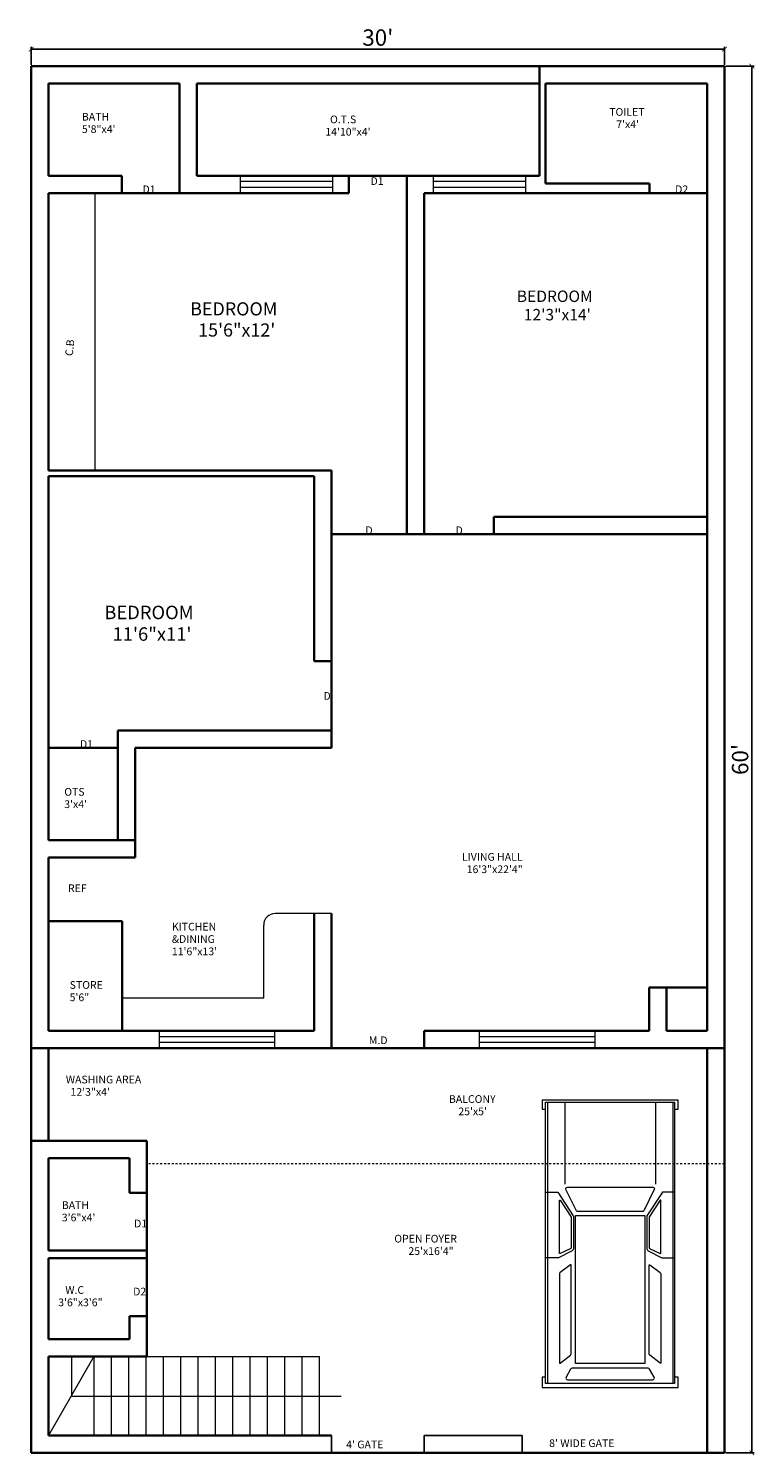
# Model space of a CAD drawing. Units: inches. Extents: x 3799 to 20199, y 1682 to 8087.
# Tile 15 of 30: x 10024 to 10401, y 5781 to 6522. Entities that reach past the tile are written whole.
import ezdxf

# ---------------------------------------------------------------- set-up
doc = ezdxf.new("R2010")
doc.units = ezdxf.units.IN
doc.linetypes.add('JIS_02_1.0', pattern=[2, 1, -1])
for name, color, linetype, lineweight in [('A-ANNO-DIMS', 2, 'Continuous', 18), ('A-ANNO-SYMB', 3, 'Continuous', 18), ('A-ANNO-TEXT', 7, 'Continuous', 18), ('A-AREA-IDEN', 7, 'Continuous', 18), ('A-FLOR-CASE', 32, 'Continuous', 18), ('A-FLOR-STRS', 41, 'Continuous', 18), ('A-GLAZ', 152, 'Continuous', 18), ('A-SITE-OVHD', 8, 'JIS_02_1.0', 18), ('A-SITE-VEHC', 8, 'Continuous', 13), ('A-WALL', 7, 'Continuous', 35), ('C-PROP', 7, 'Continuous', 25)]:
    doc.layers.add(name, color=color, linetype=linetype, lineweight=lineweight)
doc.styles.get("Standard").update_dxf_attribs({"font": 'arial.ttf'})
doc.dimstyles.new('ISO-25', dxfattribs={"dimtxt": 8.5, "dimasz": 2.5, "dimexe": 1.25, "dimexo": 0.625, "dimtad": 1, "dimdec": 0, "dimlunit": 3, "dimtxsty": 'Standard', "dimblk": 'ARCHTICK', "dimcen": 2.5, "dimadec": 0, "dimazin": 0, "dimtfac": 1, "dimtdec": 0, "dimtmove": 0, "dimatfit": 3, "dimfxl": 1, "dimarcsym": 0})

# ---------------------------------------------------------------- blocks, each defined once
blk = doc.blocks.new('_ArchTick')
at = {"color": 0, "linetype": 'ByBlock', "const_width": 0.15}
blk.add_lwpolyline([(-0.5, -0.5), (0.5, 0.5)], dxfattribs=at)
blk = doc.blocks.new('*D197')
at = {"layer": 'A-ANNO-DIMS', "color": 0, "lineweight": -2, "transparency": 16777216}
for p, q in [((10025.38, 6502.81), (10025.38, 6512.16)), ((10385.38, 6510.91), (10025.38, 6510.91)), ((10385.38, 6502.81), (10385.38, 6512.16))]:
    blk.add_line(p, q, dxfattribs=at)
at = {"layer": 'Defpoints', "color": 0, "transparency": 16777216}
for p in [(10025.38, 6510.91), (10025.38, 6502.19), (10385.38, 6502.19)]:
    blk.add_point(p, dxfattribs=at)
at = {"layer": 'A-ANNO-DIMS', "color": 0, "lineweight": -2, "transparency": 16777216, "xscale": 2.5, "yscale": 2.5, "zscale": 2.5, "rotation": 180}
blk.add_blockref('_ArchTick', (10025.38, 6510.91), dxfattribs=at)
at = {"layer": 'A-ANNO-DIMS', "color": 0, "lineweight": -2, "transparency": 16777216, "xscale": 2.5, "yscale": 2.5, "zscale": 2.5}
blk.add_blockref('_ArchTick', (10385.38, 6510.91), dxfattribs=at)
at = {"layer": 'A-ANNO-DIMS', "color": 0, "transparency": 16777216, "insert": (10205.38, 6515.88), "char_height": 8.5, "attachment_point": 5}
blk.add_mtext("30'", dxfattribs=at)
blk = doc.blocks.new('*D198')
at = {"layer": 'A-ANNO-DIMS', "color": 0, "lineweight": -2, "transparency": 16777216}
for p, q in [((10386.01, 6502.19), (10400.8, 6502.19)), ((10399.55, 5782.19), (10399.55, 6502.19)), ((10386.01, 5782.19), (10400.8, 5782.19))]:
    blk.add_line(p, q, dxfattribs=at)
at = {"layer": 'Defpoints', "color": 0, "transparency": 16777216}
for p in [(10385.38, 6502.19), (10399.55, 6502.19), (10385.38, 5782.19)]:
    blk.add_point(p, dxfattribs=at)
at = {"layer": 'A-ANNO-DIMS', "color": 0, "lineweight": -2, "transparency": 16777216, "xscale": 2.5, "yscale": 2.5, "zscale": 2.5}
for p, rotation in [((10399.55, 6502.19), 90), ((10399.55, 5782.19), 270)]:
    blk.add_blockref('_ArchTick', p, dxfattribs=dict(at, rotation=rotation))
at = {"layer": 'A-ANNO-DIMS', "color": 0, "transparency": 16777216, "insert": (10394.59, 6142.19), "char_height": 8.5, "attachment_point": 5, "rotation": 90}
blk.add_mtext("60'", dxfattribs=at)
blk = doc.blocks.new('*U199')
for p, q in [((1.28, 38.87), (175.66, 38.87)), ((1.28, 28.15), (52.13, 28.15)), ((1.28, -28.15), (52.13, -28.15)), ((1.28, -38.87), (175.66, -38.87))]:
    blk.add_line(p, q)
for points in [[(5.57, 40.01), (5.57, 42.18), (0, 42.18), (0, -42.18), (5.57, -42.18), (5.57, -40.01), (1.28, -40.01), (1.28, 40.01)], [(1.28, 40.01), (175.66, 40.01), (175.66, -40.01), (1.28, -40.01)], [(171.74, 40.01), (175.66, 40.01), (175.66, -40.01), (171.74, -40.01), (171.74, -42.18), (178.14, -42.18), (178.14, 42.18), (171.74, 42.18)], [(71.47, 21.48), (163.42, 21.48), (163.42, -21.48), (71.47, -21.48)]]:
    blk.add_lwpolyline(points, close=True)
for points in [[(57.15, 40.01), (57.15, 32.39), (71.72, 22.83, 0.086577), (72.56, 22.68), (91.59, 22.68, 0.227875), (93.54, 23.62), (97.72, 32.11), (97.72, 40.01)], [(57.15, -40.01), (57.15, -32.39), (71.72, -22.83, -0.086577), (72.56, -22.68), (91.59, -22.68, -0.227875), (93.54, -23.62), (97.72, -32.11), (97.72, -40.01)]]:
    blk.add_lwpolyline(points, format="xyb")
for points in [[(55.49, 27.42), (68.59, 20.89, -0.284287), (69.14, 19.99), (69.14, -19.99, -0.284287), (68.59, -20.89), (55.49, -27.42, -0.557284), (54.05, -26.53), (54.05, 26.53, -0.557284)], [(62.08, 30.95), (72.14, 24.35, 0.146139), (72.69, 24.18), (91.42, 24.18, 0.29766), (92.33, 24.78), (95.09, 31.05, 0.541236), (94.86, 31.41), (62.21, 31.41, 0.744989)], [(102.19, 24.58), (106.97, 31, -0.236929), (107.78, 31.41), (162.91, 31.41, -0.621576), (163.11, 31), (158.19, 24.58, -0.233368), (157.39, 24.18), (102.39, 24.18, -0.616908)], [(171.88, 27.31), (166.83, 24.47, 0.271143), (166.32, 23.6), (166.32, -23.6, 0.271143), (166.83, -24.47), (171.88, -27.31, 0.573387), (173.37, -26.44), (173.37, 26.44, 0.573387)], [(62.08, -30.95), (72.14, -24.35, -0.146139), (72.69, -24.18), (91.42, -24.18, -0.29766), (92.33, -24.78), (95.09, -31.05, -0.541236), (94.86, -31.41), (62.21, -31.41, -0.744989)], [(102.19, -24.58), (106.97, -31, 0.236929), (107.78, -31.41), (162.91, -31.41, 0.621576), (163.11, -31), (158.19, -24.58, 0.233368), (157.39, -24.18), (102.39, -24.18, 0.616908)]]:
    blk.add_lwpolyline(points, format="xyb", close=True)
blk = doc.blocks.new('WIN-48IN-9IN-FRAME')
for p, q in [((0, 0), (0, 9)), ((48, 0), (48, 9)), ((48, 6), (0, 6)), ((48, 3), (0, 3))]:
    blk.add_line(p, q)
blk = doc.blocks.new('WIN-60IN-9IN-FRAME')
for p, q in [((0, 9), (0, 0)), ((60, 9), (60, 0)), ((60, 6), (0, 6)), ((60, 3), (0, 3))]:
    blk.add_line(p, q)

msp = doc.modelspace()

# ---------------------------------------------------------------- linework, layer by layer
at = {"layer": 'A-FLOR-CASE'}
for p, q in [((10058.38, 6436.19), (10058.38, 6292.19)), ((10181.38, 6062.18), (10152.09, 6062.18)), ((10146.09, 6018.49), (10146.09, 6056.18)), ((10072.53, 6018.49), (10146.09, 6018.49))]:
    msp.add_line(p, q, dxfattribs=at)
msp.add_arc((10152.09, 6056.18), 6, 90, 180, dxfattribs=at)
at = {"layer": 'A-FLOR-STRS'}
for p, q in [((10057.88, 5832.19), (10034.38, 5791.19)), ((10046.25, 5832.19), (10046.25, 5811.65)), ((10057.88, 5832.19), (10057.88, 5791.19)), ((10066.88, 5832.19), (10066.88, 5791.19)), ((10075.88, 5832.19), (10075.88, 5791.19)), ((10084.88, 5832.19), (10084.88, 5791.19)), ((10085.38, 5832.19), (10174.88, 5832.19)), ((10093.88, 5832.19), (10093.88, 5791.19)), ((10102.88, 5832.19), (10102.88, 5791.19)), ((10111.88, 5832.19), (10111.88, 5791.19)), ((10120.88, 5832.19), (10120.88, 5791.19)), ((10129.88, 5832.19), (10129.88, 5791.19)), ((10138.88, 5832.19), (10138.88, 5791.19)), ((10147.88, 5832.19), (10147.88, 5791.19)), ((10156.88, 5832.19), (10156.88, 5791.19)), ((10165.88, 5832.19), (10165.88, 5791.19)), ((10174.88, 5832.19), (10174.88, 5791.19)), ((10046.25, 5811.65), (10186.37, 5811.65))]:
    msp.add_line(p, q, dxfattribs=at)
at = {"layer": 'A-SITE-OVHD'}
msp.add_line((10385.38, 5932.19), (10085.38, 5932.19), dxfattribs=at)
at = {"layer": 'A-WALL'}
for p, q in [((10385.38, 6502.19), (10025.38, 6502.19)), ((10025.38, 6502.19), (10025.38, 5782.19)), ((10289.38, 6502.19), (10289.38, 6445.19)), ((10385.38, 5782.19), (10385.38, 6502.19)), ((10034.38, 6493.19), (10034.38, 6445.19)), ((10102.38, 6493.19), (10034.38, 6493.19)), ((10102.38, 6493.19), (10102.38, 6436.19)), ((10111.38, 6493.19), (10111.38, 6445.19)), ((10289.38, 6493.19), (10111.38, 6493.19)), ((10376.38, 6493.19), (10292.38, 6493.19)), ((10292.38, 6445.19), (10292.38, 6493.19)), ((10376.38, 6001.19), (10376.38, 6493.19)), ((10072.38, 6445.19), (10034.38, 6445.19)), ((10072.38, 6445.19), (10072.38, 6436.19)), ((10220.38, 6445.19), (10111.38, 6445.19)), ((10190.38, 6445.19), (10190.38, 6436.19)), ((10289.38, 6445.19), (10220.38, 6445.19)), ((10220.38, 6445.19), (10220.38, 6259.19)), ((10292.38, 6445.19), (10292.38, 6441.19)), ((10346.38, 6441.19), (10292.38, 6441.19)), ((10346.38, 6436.19), (10346.38, 6441.19)), ((10034.38, 6436.19), (10034.38, 6292.19)), ((10190.38, 6436.19), (10034.38, 6436.19)), ((10376.38, 6436.19), (10229.38, 6436.19)), ((10229.38, 6259.19), (10229.38, 6436.19)), ((10181.38, 6292.19), (10034.38, 6292.19)), ((10181.38, 6292.19), (10181.38, 6148.19)), ((10181.38, 6148.19), (10181.38, 6292.19)), ((10172.38, 6289.19), (10034.38, 6289.19)), ((10034.38, 6289.19), (10034.38, 6100.19)), ((10172.38, 6289.19), (10172.38, 6193.19)), ((10376.38, 6268.19), (10265.59, 6268.19)), ((10265.59, 6268.19), (10265.59, 6259.19)), ((10376.38, 6259.19), (10181.38, 6259.19)), ((10181.38, 6193.19), (10172.38, 6193.19)), ((10181.38, 6157.19), (10070.38, 6157.19)), ((10070.38, 6157.19), (10070.38, 6100.19)), ((10070.38, 6148.19), (10034.38, 6148.19)), ((10181.38, 6148.19), (10079.38, 6148.19)), ((10079.38, 6148.19), (10079.38, 6091.19)), ((10079.38, 6100.19), (10034.38, 6100.19)), ((10079.38, 6091.19), (10034.38, 6091.19)), ((10034.38, 6091.19), (10034.38, 6001.19)), ((10172.38, 6001.19), (10172.38, 6062.18)), ((10181.38, 5992.19), (10181.38, 6062.18)), ((10072.53, 6058.19), (10034.38, 6058.19)), ((10072.53, 6058.19), (10072.53, 6001.19)), ((10346.19, 6001.19), (10346.19, 6023.69)), ((10346.19, 6023.69), (10376.38, 6023.69)), ((10355.19, 6001.19), (10355.19, 6023.69)), ((10172.38, 6001.19), (10034.38, 6001.19)), ((10229.38, 6001.19), (10346.19, 6001.19)), ((10229.38, 5992.19), (10229.38, 6001.19)), ((10355.19, 6001.19), (10376.38, 6001.19)), ((10181.38, 5992.19), (10025.38, 5992.19)), ((10034.38, 5992.19), (10034.38, 5944.19)), ((10181.38, 5992.19), (10385.38, 5992.19)), ((10376.38, 5782.19), (10376.38, 5992.19)), ((10085.38, 5944.19), (10025.38, 5944.19)), ((10085.38, 5944.19), (10085.38, 5832.19)), ((10034.38, 5935.19), (10034.38, 5887.19)), ((10076.38, 5935.19), (10034.38, 5935.19)), ((10076.38, 5935.19), (10076.38, 5917.19)), ((10085.38, 5917.19), (10076.38, 5917.19)), ((10085.38, 5887.19), (10034.38, 5887.19)), ((10085.38, 5883.19), (10034.38, 5883.19)), ((10034.38, 5883.19), (10034.38, 5841.19)), ((10085.38, 5853.19), (10076.38, 5853.19)), ((10076.38, 5853.19), (10076.38, 5841.19)), ((10076.38, 5841.19), (10034.38, 5841.19)), ((10085.38, 5832.19), (10034.38, 5832.19)), ((10034.38, 5832.19), (10034.38, 5791.19)), ((10034.38, 5791.19), (10181.38, 5791.19)), ((10025.38, 5782.19), (10385.38, 5782.19))]:
    msp.add_line(p, q, dxfattribs=at)
at = {"layer": 'C-PROP'}
for p, q in [((10181.38, 5791.19), (10181.38, 5782.19)), ((10229.38, 5791.19), (10229.38, 5782.19)), ((10229.38, 5791.19), (10280.38, 5791.19)), ((10280.38, 5791.19), (10280.38, 5782.19))]:
    msp.add_line(p, q, dxfattribs=at)

# ---------------------------------------------------------------- block references
at = {"layer": 'A-GLAZ'}
for name, p in [('WIN-48IN-9IN-FRAME', (10133.99, 6436.19)), ('WIN-48IN-9IN-FRAME', (10234.22, 6436.19)), ('WIN-60IN-9IN-FRAME', (10091.79, 5992.19)), ('WIN-60IN-9IN-FRAME', (10258.05, 5992.19))]:
    msp.add_blockref(name, p, dxfattribs=at)
at = {"layer": 'A-SITE-VEHC', "xscale": 0.8372278023160408, "yscale": 0.8372278023160408, "zscale": 0.8372278023160408, "rotation": 270}
msp.add_blockref('*U199', (10325.98, 5965.31), dxfattribs=at)

# ---------------------------------------------------------------- texts
at = {"layer": 'A-ANNO-SYMB'}
for s, rotation, p in [('D1', 0.00111, (10083.16, 6436.19)), ('D1', 0.00111, (10201.56, 6440.47)), ('D2', 0.00111, (10359.74, 6436.19)), ('C.B', 84.30671, (10046.95, 6351.5)), ('D', 0.00111, (10198.92, 6259.19)), ('D', 0.00111, (10245.7, 6259.19)), ('D', 0.00111, (10177.15, 6173.14)), ('D1', 0.00111, (10050.69, 6148.19)), ('REF', 0.00111, (10044.46, 6073.31)), ('M.D', 0.00111, (10200.71, 5994.36)), ('D1', 0.00111, (10078.8, 5899.23)), ('D2', 0.00111, (10078.3, 5863.91))]:
    msp.add_text(s, height=4, rotation=rotation, dxfattribs=at).set_placement(p)
at = {"layer": 'A-ANNO-TEXT'}
for s, p in [("4' GATE", (10188.93, 5784.51)), ("8' WIDE GATE", (10294.33, 5785.17))]:
    msp.add_text(s, height=4, rotation=0.00111, dxfattribs=at).set_placement(p)
at = {"layer": 'A-AREA-IDEN'}
for s, height, p in [('BATH', 4, (10051.71, 6473.87)), ('  O.T.S', 4, (10178.11, 6472.49)), ('TOILET', 4, (10325.51, 6476.37)), ('5\'8"x4\'', 4, (10051.71, 6467.44)), ('14\'10"x4\'', 4, (10178.11, 6466.07)), ("   7'x4'", 4, (10325.51, 6469.95)), ('BEDROOM', 6.821, (10107.92, 6372.7)), ('BEDROOM', 5.939, (10277.53, 6379.69)), ('  12\'3"x14\'', 5.9387, (10277.53, 6370.15)), ('  15\'6"x12\'', 6.8213, (10107.92, 6361.74)), ('BEDROOM', 6.985, (10063.35, 6215.01)), ('  11\'6"x11\'', 6.9847, (10063.35, 6203.79)), ('OTS', 4, (10042.56, 6123.37)), ("3'x4'", 4, (10042.56, 6116.94)), ('LIVING HALL', 4, (10249.07, 6089.59)), ('  16\'3"x22\'4"', 4, (10249.07, 6083.17)), ('KITCHEN', 4, (10098.43, 6053.36)), ('&DINING', 4, (10098.43, 6046.93)), ('11\'6"x13\'', 4, (10098.43, 6040.51)), ('STORE', 4, (10045.34, 6023.09)), ('5\'6"', 4, (10045.34, 6016.67)), ('WASHING AREA', 4, (10043.36, 5973.99)), ('  12\'3"x4\'', 4, (10043.36, 5967.57)), ('BALCONY', 4, (10242.29, 5963.87)), ("    25'x5'", 4, (10242.29, 5957.45)), ('BATH', 4, (10041.28, 5908.79)), ('3\'6"x4\'', 4, (10041.28, 5902.36)), ('OPEN FOYER', 4, (10213.91, 5891.36)), ('      25\'x16\'4"', 4, (10213.91, 5884.93)), ('   W.C', 4, (10039.41, 5864.72)), ('3\'6"x3\'6"', 4, (10039.41, 5858.29))]:
    msp.add_text(s, height=height, rotation=0.00111, dxfattribs=at).set_placement(p)

# ---------------------------------------------------------------- dimensions: what is measured, and where the dimension line sits
at = {"layer": 'A-ANNO-DIMS'}
dim = msp.add_linear_dim(base=(10025.38, 6510.91), p1=(10385.38, 6502.19), p2=(10025.38, 6502.19), dimstyle='ISO-25', override={"dimclrd": 0, "dimclre": 0, "dimclrt": 0}, dxfattribs=at)
dim.commit()
dim.dimension.update_dxf_attribs({"geometry": '*D197', "text_midpoint": (10205.38, 6515.88)})
dim = msp.add_linear_dim(base=(10399.55, 6502.19), p1=(10385.38, 5782.19), p2=(10385.38, 6502.19), angle=90, dimstyle='ISO-25', override={"dimclrd": 0, "dimclre": 0, "dimclrt": 0}, dxfattribs=at)
dim.commit()
dim.dimension.update_dxf_attribs({"geometry": '*D198', "text_midpoint": (10394.59, 6142.19)})

doc.saveas('drawing.dxf')
